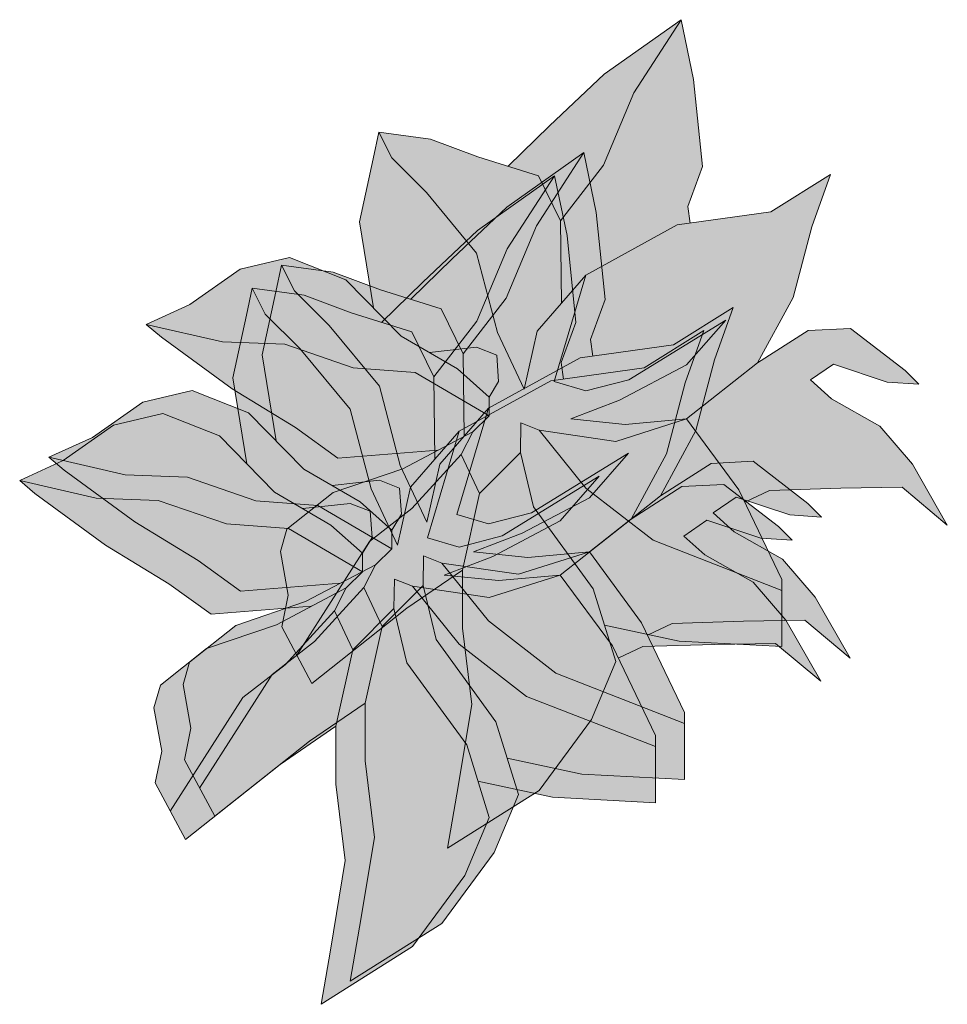
# Model space of a CAD drawing. Units: inches. Extents: x -48 to 50072, y 0 to 21068.
# Tile 75 of 75: x 44719 to 50072, y 771 to 6450. Entities that reach past the tile are written whole.
import ezdxf

# ---------------------------------------------------------------- set-up
doc = ezdxf.new("R2010")
doc.units = ezdxf.units.IN
doc.header["$MEASUREMENT"] = 0
doc.layers.add('L-PLNT', color=94, linetype='Continuous', lineweight=13)

# ---------------------------------------------------------------- blocks, each defined once
blk = doc.blocks.new('A$C1A1D2AD4')
h = blk.add_hatch(color=256)
h.set_gradient(color1=(122, 31, 0), color2=(242, 210, 28), tint=1, name='INVCYLINDER')
h.paths.add_polyline_path([(2.39, 3.6193), (2.2632, 3.8787), (1.9128, 3.9873), (1.6409, 4.0899), (1.3422, 4.1298), (1.4174, 3.9813), (1.6168, 3.7822), (1.9067, 3.4323), (2.0276, 2.9737), (2.181, 2.6481), (2.2564, 2.9818), (2.3966, 3.1433)])
h.paths.add_polyline_path([(2.8134, 4.3572), (3.0863, 4.7787), (2.6429, 4.4637), (2.3274, 4.1657), (2.088, 3.933), (2.2632, 3.8787), (2.39, 3.6193), (2.6386, 3.94)])
h = blk.add_hatch(color=256)
h.set_gradient(color1=(122, 31, 0), color2=(220, 179, 46), tint=1, name='INVCYLINDER')
h.paths.add_polyline_path([(3.1587, 4.4339), (3.0863, 4.7787), (2.8134, 4.3572), (2.6386, 3.94), (2.39, 3.6193), (2.3966, 3.1433), (2.5367, 3.3048), (3.0648, 3.5954), (3.1381, 3.6056), (3.1246, 3.7016), (3.2099, 3.9315)])
h = blk.add_hatch(color=256)
h.set_gradient(color1=(122, 31, 0), color2=(220, 179, 46), tint=1, name='INVCYLINDER')
h.paths.add_polyline_path([(1.9067, 3.4323), (1.6168, 3.7822), (1.4174, 3.9813), (1.3422, 4.1298), (1.3087, 3.9753), (1.2301, 3.6133), (1.3117, 3.1163), (1.471, 2.9538), (1.6337, 2.859), (1.9067, 2.8893), (2.0235, 2.844), (2.0336, 2.6928), (1.9794, 2.6017), (1.9794, 2.4934), (1.8844, 2.4019), (1.8167, 2.27), (1.9223, 2.0453), (2.1594, 2.2821), (2.1624, 2.4528), (2.2672, 2.4113), (2.7091, 2.3467), (3.1187, 2.4759), (2.763, 2.4436), (2.4505, 2.4759), (2.7307, 2.5835), (3.1187, 2.7881), (3.3451, 3.0464), (2.7846, 2.7019), (2.5367, 2.6373), (2.3534, 2.6912), (2.5367, 3.3048), (2.2564, 2.9818), (2.181, 2.6481), (2.0276, 2.9737)])
h = blk.add_hatch(color=256)
h.set_gradient(color1=(122, 31, 0), color2=(220, 179, 46), tint=1, name='INVCYLINDER')
h.paths.add_polyline_path([(3.8409, 3.5846), (3.9487, 3.886), (3.6038, 3.6708), (3.0648, 3.5954), (2.5367, 3.3048), (2.3534, 2.6912), (2.5367, 2.6373), (2.7846, 2.7019), (3.3451, 3.0464), (3.1187, 2.7881), (2.7307, 2.5835), (2.4505, 2.4759), (2.763, 2.4436), (3.1187, 2.4759), (3.5283, 2.7988), (3.7331, 3.1756)])
h = blk.add_hatch(color=256)
h.set_gradient(color1=(122, 31, 0), color2=(242, 210, 28), tint=1, name='INVCYLINDER')
h.paths.add_polyline_path([(1.1524, 3.2787), (0.827, 3.4074), (0.5423, 3.3397), (0.2508, 3.1366), (0, 3.0215), (0.4406, 2.9199), (0.7999, 2.9064), (1.1931, 2.771), (1.5523, 2.7439), (1.9794, 2.4934), (1.9794, 2.6017), (1.7964, 2.7642), (1.471, 2.9538)])
h.paths.add_polyline_path([(1.5523, 2.7439), (1.1931, 2.771), (0.7999, 2.9064), (0.4406, 2.9199), (0, 3.0215), (0.0881, 2.947), (0.4948, 2.6491), (0.8609, 2.4257), (1.1049, 2.2497), (1.6828, 2.2955), (1.8844, 2.4019), (1.9794, 2.4934)])
h = blk.add_hatch(color=256)
h.set_gradient(color1=(122, 31, 0), color2=(220, 179, 46), tint=1, name='INVCYLINDER')
h.paths.add_polyline_path([(3.9544, 2.5918), (3.8328, 2.701), (3.9666, 2.7921), (4.2765, 2.6889), (4.4589, 2.6767), (4.3799, 2.7557), (4.0638, 2.9985), (3.8207, 2.9863), (3.5283, 2.7988), (3.1187, 2.4759), (3.4205, 2.0668), (3.4546, 1.9959), (3.5958, 2.0637), (4.0091, 2.0758), (4.3616, 2.0819), (4.623, 1.8634), (4.4224, 2.2154), (4.234, 2.4339)])
h = blk.add_hatch(color=256)
h.set_gradient(color1=(122, 31, 0), color2=(220, 179, 46), tint=1, name='INVCYLINDER')
h.paths.add_polyline_path([(3.6685, 1.4865), (2.9247, 1.7762), (2.5367, 2.0776), (2.2672, 2.4113), (2.1624, 2.4528), (2.1594, 2.2821), (2.2349, 1.9699), (2.5798, 1.4963), (2.6445, 1.2864), (3.0756, 1.1949), (3.6685, 1.1626)])
h = blk.add_hatch(color=256)
h.set_gradient(color1=(122, 31, 0), color2=(220, 179, 46), tint=1, name='INVCYLINDER')
h.paths.add_polyline_path([(3.1187, 2.4759), (2.7091, 2.3467), (2.2672, 2.4113), (2.5367, 2.0776), (2.9247, 1.7762), (3.6685, 1.4865), (3.6685, 1.5501), (3.4205, 2.0668)])
h = blk.add_hatch(color=256)
h.set_gradient(color1=(122, 31, 0), color2=(220, 179, 46), tint=1, name='INVCYLINDER')
h.paths.add_polyline_path([(1.532, 1.9586), (1.8167, 2.27), (1.8844, 2.4019), (1.4813, 2.1892), (1.0781, 2.0525), (0.8119, 1.8398), (0.7739, 1.7106), (0.8195, 1.46), (0.7815, 1.2776), (0.869, 1.1143), (1.0982, 1.4712), (1.288, 1.7691)])
h = blk.add_hatch(color=256)
h.set_gradient(color1=(122, 31, 0), color2=(220, 179, 46), tint=1, name='INVCYLINDER')
h.paths.add_polyline_path([(2.5798, 1.4963), (2.2349, 1.9699), (2.1594, 2.2821), (1.9223, 2.0453), (1.8253, 1.6039), (1.8253, 1.2702), (1.8792, 0.8289), (1.7929, 0.3122), (1.739, 0), (2.2672, 0.3337), (2.569, 0.7428), (2.7091, 1.0765)])
h = blk.add_hatch(color=256)
h.set_gradient(color1=(122, 31, 0), color2=(220, 179, 46), tint=1, name='INVCYLINDER')
h.paths.add_polyline_path([(1.9223, 2.0453), (1.8167, 2.27), (1.532, 1.9586), (1.288, 1.7691), (1.0982, 1.4712), (0.869, 1.1143), (0.9564, 0.951), (1.5041, 1.384), (1.8253, 1.6039)])
at = {"color": 0}
for p, q in [((2.6429, 4.4637), (3.0863, 4.7787)), ((2.8134, 4.3572), (3.0863, 4.7787)), ((3.0863, 4.7787), (3.1587, 4.4339)), ((2.3274, 4.1657), (2.6429, 4.4637)), ((3.1587, 4.4339), (3.2099, 3.9315)), ((2.6386, 3.94), (2.8134, 4.3572)), ((2.088, 3.933), (2.3274, 4.1657)), ((1.3087, 3.9753), (1.3422, 4.1298)), ((1.3422, 4.1298), (1.6409, 4.0899)), ((1.4174, 3.9813), (1.3422, 4.1298)), ((1.6409, 4.0899), (1.9128, 3.9873)), ((1.2301, 3.6133), (1.3087, 3.9753)), ((1.6168, 3.7822), (1.4174, 3.9813)), ((1.9128, 3.9873), (2.2632, 3.8787)), ((2.39, 3.6193), (2.6386, 3.94)), ((3.2099, 3.9315), (3.1246, 3.7016)), ((2.2632, 3.8787), (2.39, 3.6193)), ((3.9487, 3.886), (3.6038, 3.6708)), ((3.8409, 3.5846), (3.9487, 3.886)), ((1.9067, 3.4323), (1.6168, 3.7822)), ((3.1246, 3.7016), (3.1381, 3.6056)), ((3.6038, 3.6708), (3.0648, 3.5954)), ((1.3117, 3.1163), (1.2301, 3.6133)), ((2.39, 3.6193), (2.3966, 3.1433)), ((3.0648, 3.5954), (2.5367, 3.3048)), ((3.7331, 3.1756), (3.8409, 3.5846)), ((0.5423, 3.3397), (0.827, 3.4074)), ((0.827, 3.4074), (1.1524, 3.2787)), ((2.0276, 2.9737), (1.9067, 3.4323)), ((0.2508, 3.1366), (0.5423, 3.3397)), ((2.5367, 3.3048), (2.2564, 2.9818)), ((2.5367, 3.3048), (2.3534, 2.6912)), ((1.1524, 3.2787), (1.471, 2.9538)), ((0, 3.0215), (0.2508, 3.1366)), ((3.5283, 2.7988), (3.7331, 3.1756)), ((0.0881, 2.947), (0, 3.0215)), ((0, 3.0215), (0.4406, 2.9199)), ((2.7846, 2.7019), (3.3451, 3.0464)), ((3.3451, 3.0464), (3.1187, 2.7881)), ((1.471, 2.9538), (1.7964, 2.7642)), ((2.181, 2.6481), (2.0276, 2.9737)), ((2.2564, 2.9818), (2.181, 2.6481)), ((3.5283, 2.7988), (3.8207, 2.9863)), ((3.8207, 2.9863), (4.0638, 2.9985)), ((4.0638, 2.9985), (4.3799, 2.7557)), ((0.4948, 2.6491), (0.0881, 2.947)), ((0.4406, 2.9199), (0.7999, 2.9064)), ((0.7999, 2.9064), (1.1931, 2.771)), ((1.6337, 2.859), (1.9067, 2.8893)), ((1.9067, 2.8893), (2.0235, 2.844)), ((2.0235, 2.844), (2.0336, 2.6928)), ((3.1187, 2.7881), (2.7307, 2.5835)), ((3.1187, 2.4759), (3.5283, 2.7988)), ((3.9666, 2.7921), (3.8328, 2.701)), ((4.2765, 2.6889), (3.9666, 2.7921)), ((1.1931, 2.771), (1.5523, 2.7439)), ((1.5523, 2.7439), (1.9794, 2.4934)), ((1.7964, 2.7642), (1.9794, 2.6017)), ((4.3799, 2.7557), (4.4589, 2.6767)), ((2.0336, 2.6928), (1.9794, 2.6017)), ((2.3534, 2.6912), (2.5367, 2.6373)), ((2.5367, 2.6373), (2.7846, 2.7019)), ((3.8328, 2.701), (3.9544, 2.5918)), ((4.4589, 2.6767), (4.2765, 2.6889)), ((0.8609, 2.4257), (0.4948, 2.6491)), ((1.9794, 2.4934), (1.9794, 2.6017)), ((2.7307, 2.5835), (2.4505, 2.4759)), ((3.9544, 2.5918), (4.234, 2.4339)), ((1.9794, 2.4934), (1.8844, 2.4019)), ((2.1594, 2.2821), (2.1624, 2.4528)), ((2.1624, 2.4528), (2.2672, 2.4113)), ((2.4505, 2.4759), (2.763, 2.4436)), ((3.1187, 2.4759), (2.7091, 2.3467)), ((2.763, 2.4436), (3.1187, 2.4759)), ((3.4205, 2.0668), (3.1187, 2.4759)), ((1.1049, 2.2497), (0.8609, 2.4257)), ((1.4813, 2.1892), (1.8844, 2.4019)), ((1.8167, 2.27), (1.8844, 2.4019)), ((2.2672, 2.4113), (2.5367, 2.0776)), ((2.7091, 2.3467), (2.2672, 2.4113)), ((4.234, 2.4339), (4.4224, 2.2154)), ((1.6828, 2.2955), (1.1049, 2.2497)), ((2.1594, 2.2821), (1.9223, 2.0453)), ((2.2349, 1.9699), (2.1594, 2.2821)), ((1.532, 1.9586), (1.8167, 2.27)), ((1.8167, 2.27), (1.9223, 2.0453)), ((4.4224, 2.2154), (4.623, 1.8634)), ((1.0781, 2.0525), (1.4813, 2.1892)), ((0.8119, 1.8398), (1.0781, 2.0525)), ((1.9223, 2.0453), (1.8253, 1.6039)), ((2.5367, 2.0776), (2.9247, 1.7762)), ((3.6685, 1.5501), (3.4205, 2.0668)), ((3.5958, 2.0637), (3.4546, 1.9959)), ((4.0091, 2.0758), (3.5958, 2.0637)), ((4.3616, 2.0819), (4.0091, 2.0758)), ((4.623, 1.8634), (4.3616, 2.0819)), ((1.288, 1.7691), (1.532, 1.9586)), ((2.5798, 1.4963), (2.2349, 1.9699)), ((0.7739, 1.7106), (0.8119, 1.8398)), ((1.0982, 1.4712), (1.288, 1.7691)), ((2.9247, 1.7762), (3.6685, 1.4865)), ((0.8195, 1.46), (0.7739, 1.7106)), ((1.8253, 1.6039), (1.5041, 1.384)), ((1.8253, 1.6039), (1.8253, 1.2702)), ((3.6685, 1.1626), (3.6685, 1.5501)), ((2.7091, 1.0765), (2.5798, 1.4963)), ((0.7815, 1.2776), (0.8195, 1.46)), ((0.869, 1.1143), (1.0982, 1.4712)), ((1.5041, 1.384), (0.9564, 0.951)), ((0.9564, 0.951), (0.7815, 1.2776)), ((1.8253, 1.2702), (1.8792, 0.8289)), ((2.6445, 1.2864), (3.0756, 1.1949)), ((3.0756, 1.1949), (3.6685, 1.1626)), ((2.569, 0.7428), (2.7091, 1.0765)), ((1.8792, 0.8289), (1.7929, 0.3122)), ((2.2672, 0.3337), (2.569, 0.7428)), ((1.739, 0), (2.2672, 0.3337)), ((1.7929, 0.3122), (1.739, 0))]:
    blk.add_line(p, q, dxfattribs=at)

msp = doc.modelspace()

# ---------------------------------------------------------------- block references
at = {"layer": 'L-PLNT', "xscale": 1000, "yscale": 1000, "zscale": 1000}
for p in [(45449.303, 1671.216), (44887.769, 904.321), (44718.692, 771.066)]:
    msp.add_blockref('A$C1A1D2AD4', p, dxfattribs=at)

doc.saveas('drawing.dxf')
